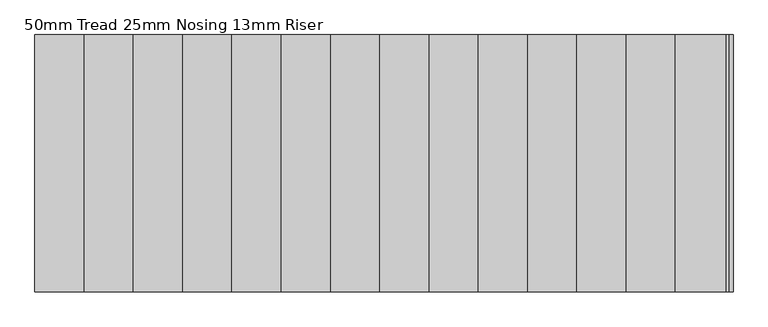
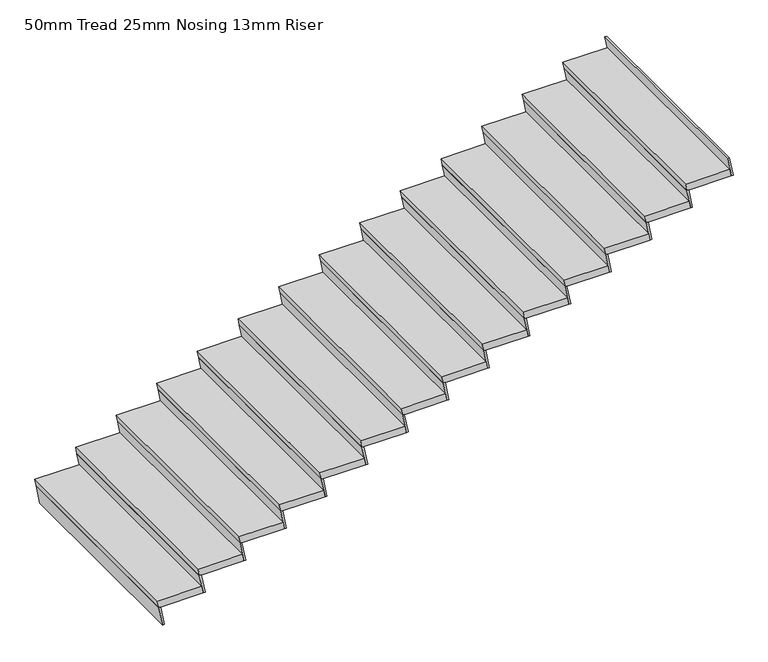
"""IFC4 building model written with IfcOpenShell, lengths in millimetres: stair flight geometry, 50mm Tread 25mm Nosing 13mm Riser."""

from ifc_helpers import new_model, si_unit, frame, origin, place, context, project, spatial, polyline, outline, extrude, source, transform, mapped, element, save


def stair_flight_50mm_tread_25mm_nosing_13mm_riser_0c3918f5(model_context):
    return source(origin(), model_context, "Body", "SweptSolid", [
        extrude(outline(polyline([(2133.3333333, 65.6033064), (2133.3333333, -234.3966936), (2083.3333333, -225.0216936), (2083.3333333, 74.9783064), (2133.3333333, 65.6033064)])), frame((0.0, 601.2300402, 0.0), z_axis=(0.0, 1.0, 0.0), x_axis=(0.0, 0.0, 1.0)), (0.0, 0.0, 1.0), 1437.199031),
        extrude(outline(polyline([(2083.3333333, -225.0216936), (1950.0, -200.0216936), (1950.0, -187.303865), (2083.3333333, -212.303865), (2083.3333333, -225.0216936)])), frame((0.0, 601.2300402, 0.0), z_axis=(0.0, 1.0, 0.0), x_axis=(0.0, 0.0, 1.0)), (0.0, 0.0, 1.0), 1437.199031),
        extrude(outline(polyline([(2216.6666667, 49.9783064), (2083.3333333, 74.9783064), (2083.3333333, 87.696135), (2216.6666667, 62.696135), (2216.6666667, 49.9783064)])), frame((0.0, 601.2300402, 0.0), z_axis=(0.0, 1.0, 0.0), x_axis=(0.0, 0.0, 1.0)), (0.0, 0.0, 1.0), 1437.199031),
        extrude(outline(polyline([(2266.6666667, 340.6033064), (2266.6666667, 40.6033064), (2216.6666667, 49.9783064), (2216.6666667, 349.9783064), (2266.6666667, 340.6033064)])), frame((0.0, 601.2300402, 0.0), z_axis=(0.0, 1.0, 0.0), x_axis=(0.0, 0.0, 1.0)), (0.0, 0.0, 1.0), 1437.199031),
        extrude(outline(polyline([(2350.0, 324.9783064), (2216.6666667, 349.9783064), (2216.6666667, 362.696135), (2350.0, 337.696135), (2350.0, 324.9783064)])), frame((0.0, 601.2300402, 0.0), z_axis=(0.0, 1.0, 0.0), x_axis=(0.0, 0.0, 1.0)), (0.0, 0.0, 1.0), 1437.199031),
        extrude(outline(polyline([(2400.0, 615.6033064), (2400.0, 315.6033064), (2350.0, 324.9783064), (2350.0, 624.9783064), (2400.0, 615.6033064)])), frame((0.0, 601.2300402, 0.0), z_axis=(0.0, 1.0, 0.0), x_axis=(0.0, 0.0, 1.0)), (0.0, 0.0, 1.0), 1437.199031),
        extrude(outline(polyline([(2483.3333333, 599.9783064), (2350.0, 624.9783064), (2350.0, 637.696135), (2483.3333333, 612.696135), (2483.3333333, 599.9783064)])), frame((0.0, 601.2300402, 0.0), z_axis=(0.0, 1.0, 0.0), x_axis=(0.0, 0.0, 1.0)), (0.0, 0.0, 1.0), 1437.199031),
        extrude(outline(polyline([(2533.3333333, 890.6033064), (2533.3333333, 590.6033064), (2483.3333333, 599.9783064), (2483.3333333, 899.9783064), (2533.3333333, 890.6033064)])), frame((0.0, 601.2300402, 0.0), z_axis=(0.0, 1.0, 0.0), x_axis=(0.0, 0.0, 1.0)), (0.0, 0.0, 1.0), 1437.199031),
        extrude(outline(polyline([(2616.6666667, 874.9783064), (2483.3333333, 899.9783064), (2483.3333333, 912.696135), (2616.6666667, 887.696135), (2616.6666667, 874.9783064)])), frame((0.0, 601.2300402, 0.0), z_axis=(0.0, 1.0, 0.0), x_axis=(0.0, 0.0, 1.0)), (0.0, 0.0, 1.0), 1437.199031),
        extrude(outline(polyline([(2666.6666667, 1165.6033064), (2666.6666667, 865.6033064), (2616.6666667, 874.9783064), (2616.6666667, 1174.9783064), (2666.6666667, 1165.6033064)])), frame((0.0, 601.2300402, 0.0), z_axis=(0.0, 1.0, 0.0), x_axis=(0.0, 0.0, 1.0)), (0.0, 0.0, 1.0), 1437.199031),
        extrude(outline(polyline([(2750.0, 1149.9783064), (2616.6666667, 1174.9783064), (2616.6666667, 1187.696135), (2750.0, 1162.696135), (2750.0, 1149.9783064)])), frame((0.0, 601.2300402, 0.0), z_axis=(0.0, 1.0, 0.0), x_axis=(0.0, 0.0, 1.0)), (0.0, 0.0, 1.0), 1437.199031),
        extrude(outline(polyline([(2800.0, 1440.6033064), (2800.0, 1140.6033064), (2750.0, 1149.9783064), (2750.0, 1449.9783064), (2800.0, 1440.6033064)])), frame((0.0, 601.2300402, 0.0), z_axis=(0.0, 1.0, 0.0), x_axis=(0.0, 0.0, 1.0)), (0.0, 0.0, 1.0), 1437.199031),
        extrude(outline(polyline([(2883.3333333, 1424.9783064), (2750.0, 1449.9783064), (2750.0, 1462.696135), (2883.3333333, 1437.696135), (2883.3333333, 1424.9783064)])), frame((0.0, 601.2300402, 0.0), z_axis=(0.0, 1.0, 0.0), x_axis=(0.0, 0.0, 1.0)), (0.0, 0.0, 1.0), 1437.199031),
        extrude(outline(polyline([(2933.3333333, 1715.6033064), (2933.3333333, 1415.6033064), (2883.3333333, 1424.9783064), (2883.3333333, 1724.9783064), (2933.3333333, 1715.6033064)])), frame((0.0, 601.2300402, 0.0), z_axis=(0.0, 1.0, 0.0), x_axis=(0.0, 0.0, 1.0)), (0.0, 0.0, 1.0), 1437.199031),
        extrude(outline(polyline([(3016.6666667, 1699.9783064), (2883.3333333, 1724.9783064), (2883.3333333, 1737.696135), (3016.6666667, 1712.696135), (3016.6666667, 1699.9783064)])), frame((0.0, 601.2300402, 0.0), z_axis=(0.0, 1.0, 0.0), x_axis=(0.0, 0.0, 1.0)), (0.0, 0.0, 1.0), 1437.199031),
        extrude(outline(polyline([(3066.6666667, 1990.6033064), (3066.6666667, 1690.6033064), (3016.6666667, 1699.9783064), (3016.6666667, 1999.9783064), (3066.6666667, 1990.6033064)])), frame((0.0, 601.2300402, 0.0), z_axis=(0.0, 1.0, 0.0), x_axis=(0.0, 0.0, 1.0)), (0.0, 0.0, 1.0), 1437.199031),
        extrude(outline(polyline([(3150.0, 1974.9783064), (3016.6666667, 1999.9783064), (3016.6666667, 2012.696135), (3150.0, 1987.696135), (3150.0, 1974.9783064)])), frame((0.0, 601.2300402, 0.0), z_axis=(0.0, 1.0, 0.0), x_axis=(0.0, 0.0, 1.0)), (0.0, 0.0, 1.0), 1437.199031),
        extrude(outline(polyline([(3200.0, 2265.6033064), (3200.0, 1965.6033064), (3150.0, 1974.9783064), (3150.0, 2274.9783064), (3200.0, 2265.6033064)])), frame((0.0, 601.2300402, 0.0), z_axis=(0.0, 1.0, 0.0), x_axis=(0.0, 0.0, 1.0)), (0.0, 0.0, 1.0), 1437.199031),
        extrude(outline(polyline([(3283.3333333, 2249.9783064), (3150.0, 2274.9783064), (3150.0, 2287.696135), (3283.3333333, 2262.696135), (3283.3333333, 2249.9783064)])), frame((0.0, 601.2300402, 0.0), z_axis=(0.0, 1.0, 0.0), x_axis=(0.0, 0.0, 1.0)), (0.0, 0.0, 1.0), 1437.199031),
        extrude(outline(polyline([(3333.3333333, 2540.6033064), (3333.3333333, 2240.6033064), (3283.3333333, 2249.9783064), (3283.3333333, 2549.9783064), (3333.3333333, 2540.6033064)])), frame((0.0, 601.2300402, 0.0), z_axis=(0.0, 1.0, 0.0), x_axis=(0.0, 0.0, 1.0)), (0.0, 0.0, 1.0), 1437.199031),
        extrude(outline(polyline([(3416.6666667, 2524.9783064), (3283.3333333, 2549.9783064), (3283.3333333, 2562.696135), (3416.6666667, 2537.696135), (3416.6666667, 2524.9783064)])), frame((0.0, 601.2300402, 0.0), z_axis=(0.0, 1.0, 0.0), x_axis=(0.0, 0.0, 1.0)), (0.0, 0.0, 1.0), 1437.199031),
        extrude(outline(polyline([(3466.6666667, 2815.6033064), (3466.6666667, 2515.6033064), (3416.6666667, 2524.9783064), (3416.6666667, 2824.9783064), (3466.6666667, 2815.6033064)])), frame((0.0, 601.2300402, 0.0), z_axis=(0.0, 1.0, 0.0), x_axis=(0.0, 0.0, 1.0)), (0.0, 0.0, 1.0), 1437.199031),
        extrude(outline(polyline([(3550.0, 2799.9783064), (3416.6666667, 2824.9783064), (3416.6666667, 2837.696135), (3550.0, 2812.696135), (3550.0, 2799.9783064)])), frame((0.0, 601.2300402, 0.0), z_axis=(0.0, 1.0, 0.0), x_axis=(0.0, 0.0, 1.0)), (0.0, 0.0, 1.0), 1437.199031),
        extrude(outline(polyline([(3600.0, 3090.6033064), (3600.0, 2790.6033064), (3550.0, 2799.9783064), (3550.0, 3099.9783064), (3600.0, 3090.6033064)])), frame((0.0, 601.2300402, 0.0), z_axis=(0.0, 1.0, 0.0), x_axis=(0.0, 0.0, 1.0)), (0.0, 0.0, 1.0), 1437.199031),
        extrude(outline(polyline([(3683.3333333, 3074.9783064), (3550.0, 3099.9783064), (3550.0, 3112.696135), (3683.3333333, 3087.696135), (3683.3333333, 3074.9783064)])), frame((0.0, 601.2300402, 0.0), z_axis=(0.0, 1.0, 0.0), x_axis=(0.0, 0.0, 1.0)), (0.0, 0.0, 1.0), 1437.199031),
        extrude(outline(polyline([(3733.3333333, 3365.6033064), (3733.3333333, 3065.6033064), (3683.3333333, 3074.9783064), (3683.3333333, 3374.9783064), (3733.3333333, 3365.6033064)])), frame((0.0, 601.2300402, 0.0), z_axis=(0.0, 1.0, 0.0), x_axis=(0.0, 0.0, 1.0)), (0.0, 0.0, 1.0), 1437.199031),
        extrude(outline(polyline([(3816.6666667, 3349.9783064), (3683.3333333, 3374.9783064), (3683.3333333, 3387.696135), (3816.6666667, 3362.696135), (3816.6666667, 3349.9783064)])), frame((0.0, 601.2300402, 0.0), z_axis=(0.0, 1.0, 0.0), x_axis=(0.0, 0.0, 1.0)), (0.0, 0.0, 1.0), 1437.199031),
        extrude(outline(polyline([(3950.0, 3624.9783064), (3816.6666667, 3649.9783064), (3816.6666667, 3662.696135), (3950.0, 3637.696135), (3950.0, 3624.9783064)])), frame((0.0, 601.2300402, 0.0), z_axis=(0.0, 1.0, 0.0), x_axis=(0.0, 0.0, 1.0)), (0.0, 0.0, 1.0), 1437.199031),
        extrude(outline(polyline([(3866.6666667, 3640.6033064), (3866.6666667, 3340.6033064), (3816.6666667, 3349.9783064), (3816.6666667, 3649.9783064), (3866.6666667, 3640.6033064)])), frame((0.0, 601.2300402, 0.0), z_axis=(0.0, 1.0, 0.0), x_axis=(0.0, 0.0, 1.0)), (0.0, 0.0, 1.0), 1437.199031),
    ])


if __name__ == "__main__":
    model = new_model("IFC4")
    model_context = context("Model", 3, world=origin())
    ifc_project = project(units=[si_unit("LENGTHUNIT", "METRE", prefix="MILLI")], contexts=[model_context])
    site = spatial("IfcSite", under=ifc_project)
    building = spatial("IfcBuilding", under=site)
    placement = place(None, origin())
    stair_flight_50mm_tread_25mm_nosing_13mm_riser_shape = stair_flight_50mm_tread_25mm_nosing_13mm_riser_0c3918f5(model_context)
    element("IfcStairFlight", 1, ObjectType="50mm Tread 25mm Nosing 13mm Riser", at=placement, inside=building, context=model_context, shape_type="MappedRepresentation", body=[
        mapped(stair_flight_50mm_tread_25mm_nosing_13mm_riser_shape, transform((0.0, 0.0, 0.0), x_axis=(1.0, 0.0, 0.0), y_axis=(0.0, 1.0, 0.0), z_axis=(0.0, 0.0, 1.0))),
    ])
    save(model, "model.ifc")
